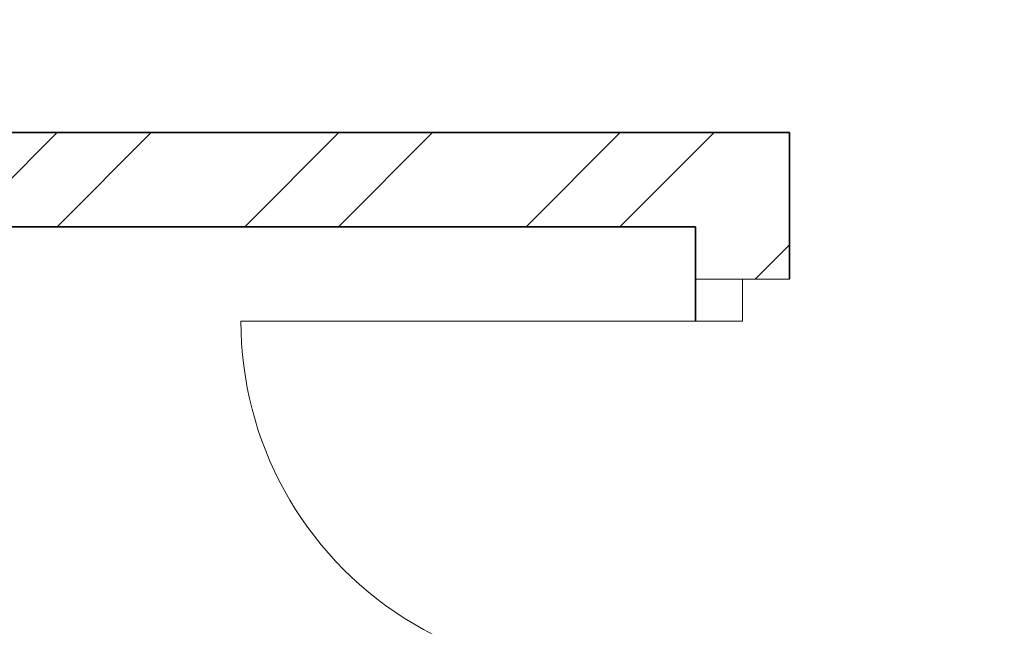
# Model space of a CAD drawing. Units: inches. Extents: x 1885 to 2748, y 783 to 2421.
# Tile 45 of 117: x 2192 to 2240, y 1591 to 1620. Entities that reach past the tile are written whole.
import ezdxf

# ---------------------------------------------------------------- set-up
doc = ezdxf.new("R2010")
doc.units = ezdxf.units.IN
doc.layers.add('A-DOOR', color=31, linetype='Continuous', lineweight=18)
doc.layers.add('A-WALL', color=7, linetype='Continuous', lineweight=35)
doc.layers.add('A-WALL-PATT', color=85, linetype='Continuous', lineweight=13, true_color=0x58ba48)

msp = doc.modelspace()

# ---------------------------------------------------------------- hatches: boundary and pattern name
at = {"layer": 'A-WALL-PATT'}
h = msp.add_hatch(dxfattribs=at)
h.set_pattern_fill('ANSI32', color=256)
h.paths.add_polyline_path([(2007.772, 2318.006), (1980.774, 2318.006), (1980.774, 2281.215), (1985.274, 2281.215), (1985.274, 2313.506), (2007.772, 2313.506), (2007.772, 2315.756)])
h.paths.add_polyline_path([(2094.324, 2318.006), (2067.772, 2318.006), (2067.772, 2313.506), (2094.324, 2313.506), (2094.324, 2315.756)])
h.paths.add_polyline_path([(2131.367, 2315.756), (2131.367, 2318.006), (2131.189, 2318.006), (2112.609, 2318.006), (2112.609, 2313.506), (2117.274, 2313.506), (2117.274, 2255.201), (2121.774, 2255.201), (2121.774, 2313.506), (2131.367, 2313.506)])
h.paths.add_polyline_path([(2190.512, 2318.006), (2155.367, 2318.006), (2155.367, 2313.506), (2169.774, 2313.506), (2169.774, 2229.506), (2121.774, 2229.506), (2121.774, 2233.451), (2119.524, 2233.451), (2117.274, 2233.451), (2117.274, 2201.101), (2121.774, 2201.101), (2121.774, 2225.006), (2169.774, 2225.006), (2169.774, 2165.006), (2306.274, 2165.006), (2306.274, 2066.006), (2310.774, 2066.006), (2344.274, 2066.006), (2486.274, 2066.006), (2486.274, 1886.006), (2483.02, 1886.006), (2483.02, 1881.506), (2486.274, 1881.506), (2486.274, 1880.678), (2490.774, 1880.678), (2490.774, 2070.506), (2344.274, 2070.506), (2310.774, 2070.506), (2310.774, 2165.006), (2310.774, 2173.636), (2308.524, 2173.636), (2306.274, 2173.636), (2306.274, 2169.506), (2174.274, 2169.506), (2174.274, 2313.506), (2190.512, 2313.506), (2190.512, 2315.756)])
h.paths.add_polyline_path([(1985.274, 2221.215), (1980.774, 2221.215), (1980.774, 2165.006), (1992.774, 2165.006), (1992.774, 2141.927), (1997.274, 2141.927), (1997.274, 2165.006), (2117.274, 2165.006), (2117.274, 2163.126), (2121.774, 2163.126), (2121.774, 2172.734), (2119.524, 2172.734), (2117.274, 2172.734), (2117.274, 2169.506), (1985.274, 2169.506)])
h.paths.add_polyline_path([(1997.274, 2105.927), (1992.774, 2105.927), (1992.774, 2070.506), (2016.774, 2070.506), (2016.774, 2059.123), (2019.024, 2059.123), (2021.274, 2059.123), (2021.274, 2070.506), (2117.274, 2070.506), (2117.274, 2022.506), (2114.423, 2022.506), (2114.423, 2018.006), (2123.627, 2018.006), (2123.627, 2020.256), (2123.627, 2022.506), (2121.774, 2022.506), (2121.774, 2142.587), (2119.524, 2142.587), (2117.274, 2142.587), (2117.274, 2075.006), (1997.274, 2075.006)])
h.paths.add_polyline_path([(2092.029, 2020.256), (2092.029, 2022.506), (2021.274, 2022.506), (2021.274, 2035.123), (2016.774, 2035.123), (2016.774, 2018.006), (2016.774, 1978.784), (2021.274, 1978.784), (2021.274, 2018.006), (2092.029, 2018.006)])
h.paths.add_polyline_path([(2260.938, 2022.506), (2153.105, 2022.506), (2153.105, 2020.256), (2153.105, 2018.006), (2155.274, 2018.006), (2155.274, 1886.006), (2107.629, 1886.006), (2107.629, 1881.506), (2182.911, 1881.506), (2182.911, 1883.756), (2182.911, 1886.006), (2159.774, 1886.006), (2159.774, 2018.006), (2260.938, 2018.006), (2260.938, 2020.256)])
h.paths.add_polyline_path([(2047.629, 1883.756), (2047.629, 1886.006), (2021.274, 1886.006), (2021.274, 1918.784), (2019.024, 1918.784), (2016.774, 1918.784), (2016.774, 1881.506), (2047.629, 1881.506)])
h.paths.add_polyline_path([(2306.361, 1883.756), (2306.361, 1886.006), (2296.274, 1886.006), (2296.274, 1982.006), (2316.535, 1982.006), (2316.535, 1984.256), (2316.535, 1986.506), (2296.274, 1986.506), (2296.274, 2022.506), (2289.276, 2022.506), (2289.276, 2018.006), (2291.774, 2018.006), (2291.774, 1886.006), (2242.911, 1886.006), (2242.911, 1881.506), (2306.361, 1881.506)], flags=17)
h.paths.add_polyline_path([(1985.274, 1843.006), (2021.6, 1843.006), (2021.534, 1845.441), (2021.477, 1847.506), (1980.774, 1847.506), (1980.774, 1809.446), (1985.274, 1809.446)])
h.paths.add_polyline_path([(2131.482, 1845.256), (2131.482, 1847.506), (2081.534, 1847.506), (2081.534, 1843.006), (2117.274, 1843.006), (2117.274, 1784.147), (2119.524, 1784.147), (2121.774, 1784.147), (2121.774, 1843.006), (2131.482, 1843.006)])
h.paths.add_polyline_path([(2203.886, 1847.506), (2155.482, 1847.506), (2155.482, 1843.006), (2169.774, 1843.006), (2169.774, 1759.006), (2121.774, 1759.006), (2121.774, 1761.457), (2117.274, 1761.457), (2117.274, 1730.429), (2121.774, 1730.429), (2121.774, 1754.506), (2177.421, 1754.506), (2177.421, 1756.756), (2177.421, 1759.006), (2174.274, 1759.006), (2174.274, 1843.006), (2203.886, 1843.006)])
h.paths.add_polyline_path([(2335.554, 1845.256), (2335.554, 1847.506), (2239.886, 1847.506), (2239.886, 1843.006), (2306.274, 1843.006), (2306.274, 1759.006), (2199.486, 1759.006), (2199.486, 1754.506), (2310.774, 1754.506), (2310.774, 1843.006), (2335.554, 1843.006)])
h.paths.add_polyline_path([(2348.774, 2022.506), (2344.274, 2022.506), (2344.274, 1986.506), (2341.681, 1986.506), (2341.681, 1982.006), (2344.274, 1982.006), (2344.274, 1886.006), (2330.361, 1886.006), (2330.361, 1881.506), (2361.627, 1881.506), (2361.627, 1883.756), (2361.627, 1886.006), (2348.774, 1886.006)], flags=17)
h.paths.add_polyline_path([(2283.251, 2315.756), (2283.251, 2318.006), (2238.512, 2318.006), (2238.512, 2313.506), (2283.251, 2313.506)], flags=17)
h.paths.add_polyline_path([(2363.274, 2348.006), (2388.677, 2348.006), (2388.677, 2350.256), (2388.677, 2352.506), (2358.774, 2352.506), (2358.774, 2348.006), (2358.774, 2318.006), (2344.481, 2318.006), (2344.481, 2313.506), (2358.774, 2313.506), (2358.774, 2229.506), (2310.774, 2229.506), (2310.774, 2231.952), (2306.274, 2231.952), (2306.274, 2205.611), (2310.774, 2205.611), (2310.774, 2225.006), (2358.774, 2225.006), (2358.774, 2211.506), (2452.329, 2211.506), (2452.329, 2213.756), (2452.329, 2216.006), (2363.274, 2216.006), (2363.274, 2318.006)])
h.paths.add_polyline_path([(2310.774, 2313.506), (2320.481, 2313.506), (2320.481, 2315.756), (2320.481, 2318.006), (2302.728, 2318.006), (2302.728, 2313.506), (2306.274, 2313.506), (2306.274, 2251.076), (2310.774, 2251.076)], flags=17)
h.paths.add_polyline_path([(2490.774, 2352.506), (2486.274, 2352.506), (2448.677, 2352.506), (2448.677, 2348.006), (2486.274, 2348.006), (2486.274, 2318.006), (2486.274, 2216.006), (2481.78, 2216.006), (2481.78, 2211.506), (2486.274, 2211.506), (2486.274, 2165.006), (2493.289, 2165.006), (2493.289, 2167.256), (2493.289, 2169.506), (2490.774, 2169.506), (2490.774, 2313.506), (2494.429, 2313.506), (2494.429, 2318.006), (2490.774, 2318.006)])
h.paths.add_polyline_path([(2534.653, 2318.006), (2515.691, 2318.006), (2515.691, 2313.506), (2534.653, 2313.506), (2534.653, 2315.756)])
h.paths.add_polyline_path([(2618.274, 2318.006), (2594.653, 2318.006), (2594.653, 2313.506), (2613.774, 2313.506), (2613.774, 2281.706), (2618.274, 2281.706)])
h.paths.add_polyline_path([(2618.274, 2221.706), (2613.774, 2221.706), (2613.774, 2169.506), (2554.019, 2169.506), (2554.019, 2165.006), (2613.774, 2165.006), (2613.774, 2152.878), (2618.274, 2152.878)])
h.paths.add_polyline_path([(2618.274, 2128.878), (2616.024, 2128.878), (2613.774, 2128.878), (2613.774, 2117.006), (2529.774, 2117.006), (2529.774, 2165.006), (2532.848, 2165.006), (2532.848, 2169.506), (2522.867, 2169.506), (2522.867, 2165.006), (2525.274, 2165.006), (2525.274, 2117.006), (2525.274, 2112.506), (2525.274, 2108.576), (2529.774, 2108.576), (2529.774, 2112.506), (2613.774, 2112.506), (2613.774, 2080.19), (2618.274, 2080.19)])
h.paths.add_polyline_path([(2618.274, 2044.19), (2616.024, 2044.19), (2613.774, 2044.19), (2613.774, 2015.506), (2529.774, 2015.506), (2529.774, 2088.582), (2527.524, 2088.582), (2525.274, 2088.582), (2525.274, 2011.006), (2613.774, 2011.006), (2613.774, 1956.755), (2618.274, 1956.755)])
h.paths.add_polyline_path([(2618.274, 1881.506), (2618.274, 1896.755), (2613.774, 1896.755), (2613.774, 1881.506), (2613.774, 1847.506), (2592.715, 1847.506), (2592.715, 1843.006), (2613.774, 1843.006), (2613.774, 1765.006), (2613.774, 1760.506), (2609.621, 1760.506), (2609.621, 1756.006), (2613.774, 1756.006), (2613.774, 1660.006), (2608.544, 1660.006), (2608.544, 1655.506), (2613.774, 1655.506), (2613.774, 1508.158), (2618.274, 1508.158)])
h.paths.add_polyline_path([(2565.774, 1843.006), (2568.997, 1843.006), (2568.997, 1847.506), (2490.774, 1847.506), (2490.774, 1849.7), (2488.524, 1849.7), (2486.274, 1849.7), (2486.274, 1847.506), (2477.274, 1847.506), (2477.274, 1838.506), (2477.274, 1821.493), (2486.274, 1821.493), (2486.274, 1838.506), (2561.274, 1838.506), (2561.274, 1765.006), (2486.274, 1765.006), (2486.274, 1786.157), (2477.274, 1786.157), (2477.274, 1765.006), (2477.274, 1756.006), (2486.274, 1756.006), (2565.774, 1756.006), (2585.621, 1756.006), (2585.621, 1758.256), (2585.621, 1760.506), (2565.774, 1760.506), (2565.774, 1765.006)])
h.paths.add_polyline_path([(2486.274, 1651.006), (2561.274, 1651.006), (2561.274, 1567.006), (2486.274, 1567.006), (2486.274, 1591.321), (2477.274, 1591.321), (2477.274, 1567.006), (2477.274, 1558.006), (2477.274, 1555.439), (2481.774, 1555.439), (2481.774, 1558.006), (2568.653, 1558.006), (2568.653, 1560.256), (2568.653, 1562.506), (2565.774, 1562.506), (2565.774, 1655.506), (2584.544, 1655.506), (2584.544, 1657.756), (2584.544, 1660.006), (2565.774, 1660.006), (2486.274, 1660.006), (2477.274, 1660.006), (2477.274, 1651.006), (2477.274, 1632.989), (2486.274, 1632.989)])
h.paths.add_polyline_path([(2449.967, 1883.756), (2449.967, 1886.006), (2421.627, 1886.006), (2421.627, 1881.506), (2449.967, 1881.506)], flags=17)
h.paths.add_polyline_path([(2447.274, 1847.506), (2395.554, 1847.506), (2395.554, 1843.006), (2442.774, 1843.006), (2442.774, 1809.27), (2447.274, 1809.27)])
h.paths.add_polyline_path([(1985.274, 1749.446), (1980.774, 1749.446), (1980.774, 1694.504), (1985.274, 1694.504), (1985.274, 1694.506), (1986.897, 1694.506), (1986.897, 1697.78), (1986.897, 1699.006), (1985.274, 1699.006)])
h.paths.add_polyline_path([(2152.774, 1699.006), (2121.774, 1699.006), (2121.774, 1703.668), (2119.524, 1703.668), (2117.274, 1703.668), (2117.274, 1699.006), (2009.219, 1699.006), (2009.219, 1694.506), (2148.274, 1694.506), (2148.274, 1692.631), (2152.774, 1692.631)])
h.paths.add_polyline_path([(2016.274, 1694.506), (2011.774, 1694.506), (2011.774, 1558.006), (2040.806, 1558.006), (2040.806, 1560.256), (2040.806, 1562.506), (2016.274, 1562.506)])
h.paths.add_polyline_path([(2152.774, 1663.017), (2150.524, 1663.017), (2148.274, 1663.017), (2148.274, 1562.506), (2100.806, 1562.506), (2100.806, 1558.006), (2165.119, 1558.006), (2165.119, 1560.256), (2165.119, 1562.506), (2152.774, 1562.506), (2152.774, 1610.506), (2224.774, 1610.506), (2224.774, 1607.99), (2229.274, 1607.99), (2229.274, 1615.006), (2152.774, 1615.006)])
h.paths.add_polyline_path([(2238.613, 1560.256), (2238.613, 1562.506), (2229.274, 1562.506), (2229.274, 1588.756), (2227.024, 1588.763), (2224.774, 1588.771), (2224.774, 1562.506), (2189.119, 1562.506), (2189.119, 1558.006), (2238.613, 1558.006)])
h.paths.add_polyline_path([(2336.024, 1560.256), (2336.024, 1562.506), (2310.774, 1562.506), (2310.774, 1656.347), (2308.524, 1656.347), (2306.274, 1656.347), (2306.274, 1562.506), (2286.613, 1562.506), (2286.613, 1558.006), (2336.024, 1558.006)])
h.paths.add_polyline_path([(2447.274, 1690.968), (2445.024, 1690.968), (2442.774, 1690.968), (2442.774, 1687.006), (2306.274, 1687.006), (2306.274, 1680.75), (2310.774, 1680.75), (2310.774, 1682.506), (2442.774, 1682.506), (2442.774, 1562.506), (2396.024, 1562.506), (2396.024, 1558.006), (2447.274, 1558.006)])
h.paths.add_polyline_path([(2447.274, 1749.27), (2445.024, 1749.27), (2442.774, 1749.27), (2442.774, 1717.232), (2447.274, 1717.232)])
h.paths.add_polyline_path([(2044.674, 1521.756), (2044.674, 1524.006), (2007.274, 1524.006), (2007.274, 1503.49), (2009.524, 1503.49), (2011.774, 1503.49), (2011.774, 1519.506), (2044.674, 1519.506)])
h.paths.add_polyline_path([(2177.969, 1521.756), (2177.969, 1524.006), (2104.674, 1524.006), (2104.674, 1519.506), (2145.774, 1519.506), (2145.774, 1387.506), (2143.37, 1387.506), (2143.37, 1383.006), (2251.585, 1383.006), (2251.585, 1385.256), (2251.585, 1387.506), (2150.274, 1387.506), (2150.274, 1519.506), (2177.969, 1519.506)])
h.paths.add_polyline_path([(2298.704, 1524.006), (2237.969, 1524.006), (2237.969, 1519.506), (2282.274, 1519.506), (2282.274, 1387.506), (2279.683, 1387.506), (2279.683, 1383.006), (2286.774, 1383.006), (2286.774, 1419.006), (2312.451, 1419.006), (2312.451, 1421.256), (2312.451, 1423.506), (2286.774, 1423.506), (2286.774, 1519.506), (2298.704, 1519.506), (2298.704, 1521.722)], flags=17)
h.paths.add_polyline_path([(2361.897, 1521.756), (2361.897, 1524.006), (2322.704, 1524.006), (2322.704, 1519.506), (2334.774, 1519.506), (2334.774, 1423.506), (2331.93, 1423.506), (2331.93, 1419.006), (2334.774, 1419.006), (2334.774, 1387.506), (2334.774, 1383.228), (2339.274, 1383.228), (2339.274, 1387.506), (2339.274, 1519.506), (2361.897, 1519.506)], flags=17)
h.paths.add_polyline_path([(2447.274, 1521.756), (2447.274, 1524.006), (2421.897, 1524.006), (2421.897, 1519.506), (2447.274, 1519.506)], flags=17)
h.paths.add_polyline_path([(2481.774, 1529.6), (2479.524, 1529.6), (2477.274, 1529.6), (2477.274, 1524.006), (2474.489, 1524.006), (2474.489, 1519.506), (2477.274, 1519.506), (2477.274, 1334.506), (2296.774, 1334.506), (2296.774, 1240.506), (2160.274, 1240.506), (2160.274, 1180.506), (2112.274, 1180.506), (2112.274, 1207.692), (2110.024, 1207.692), (2107.774, 1207.692), (2107.774, 1171.609), (2112.274, 1171.609), (2112.274, 1176.006), (2160.274, 1176.006), (2160.274, 1092.006), (2144.221, 1092.006), (2144.221, 1087.506), (2189.497, 1087.506), (2189.497, 1089.756), (2189.497, 1092.006), (2164.774, 1092.006), (2164.774, 1236.006), (2296.774, 1236.006), (2296.774, 1231.912), (2301.274, 1231.912), (2301.274, 1330.006), (2481.774, 1330.006), (2481.774, 1387.506)])
h.paths.add_polyline_path([(2618.274, 1448.158), (2613.774, 1448.158), (2613.774, 1382.506), (2529.774, 1382.506), (2525.274, 1382.506), (2525.274, 1307.062), (2529.774, 1307.062), (2529.774, 1378.006), (2613.774, 1378.006), (2613.774, 1354.988), (2618.274, 1354.988)])
h.paths.add_polyline_path([(2618.274, 1318.988), (2613.774, 1318.988), (2613.774, 1281.006), (2529.774, 1281.006), (2529.774, 1283.786), (2527.524, 1283.786), (2525.274, 1283.786), (2525.274, 1228.506), (2516.794, 1228.506), (2516.794, 1224.006), (2533.484, 1224.006), (2533.484, 1226.256), (2533.484, 1228.506), (2529.774, 1228.506), (2529.774, 1276.506), (2613.774, 1276.506), (2613.774, 1266.02), (2618.274, 1266.02)])
h.paths.add_polyline_path([(2618.274, 1134.964), (2613.774, 1134.964), (2613.774, 1092.006), (2594.545, 1092.006), (2594.545, 1087.506), (2618.274, 1087.506)])
h.paths.add_polyline_path([(2534.545, 1092.006), (2509.765, 1092.006), (2509.765, 1087.506), (2534.545, 1087.506), (2534.545, 1089.756)])
h.paths.add_polyline_path([(2481.274, 1224.006), (2484.117, 1224.006), (2484.117, 1226.256), (2484.117, 1228.506), (2476.774, 1228.506), (2476.774, 1198.506), (2471.61, 1198.506), (2471.61, 1194.006), (2476.774, 1194.006), (2476.774, 1062.006), (2436.894, 1062.006), (2436.894, 1057.506), (2476.774, 1057.506), (2481.274, 1057.506), (2481.274, 1062.006), (2481.274, 1087.506), (2485.354, 1087.506), (2485.354, 1089.756), (2485.354, 1092.006), (2481.274, 1092.006), (2481.274, 1117.506)])
h.paths.add_polyline_path([(2439.898, 1198.506), (2349.274, 1198.506), (2349.274, 1194.006), (2349.274, 1180.506), (2301.274, 1180.506), (2301.274, 1201.896), (2299.024, 1201.896), (2296.774, 1201.896), (2296.774, 1172.335), (2299.024, 1172.335), (2301.274, 1172.335), (2301.274, 1176.006), (2349.274, 1176.006), (2349.274, 1092.006), (2334.452, 1092.006), (2334.452, 1087.506), (2349.274, 1087.506), (2349.274, 1057.506), (2353.774, 1057.506), (2376.894, 1057.506), (2376.894, 1059.756), (2376.894, 1062.006), (2353.774, 1062.006), (2353.774, 1087.506), (2353.774, 1180.506), (2353.774, 1194.006), (2439.898, 1194.006), (2439.898, 1196.256)])
h.paths.add_polyline_path([(2270.596, 1089.756), (2270.596, 1092.006), (2249.497, 1092.006), (2249.497, 1087.506), (2270.596, 1087.506)], flags=17)
h.paths.add_polyline_path([(2310.452, 1092.006), (2301.274, 1092.006), (2301.274, 1153.292), (2296.774, 1153.292), (2296.774, 1092.006), (2293.786, 1092.006), (2293.786, 1087.506), (2310.452, 1087.506), (2310.452, 1089.756)], flags=17)
h.paths.add_polyline_path([(2112.274, 1150.328), (2110.024, 1150.328), (2107.774, 1150.328), (2107.774, 1092.006), (2104.465, 1092.006), (2104.465, 1087.506), (2120.221, 1087.506), (2120.221, 1089.756), (2120.221, 1092.006), (2112.274, 1092.006)])
h.paths.add_polyline_path([(2082.172, 1092.006), (2058.144, 1092.006), (2058.144, 1087.506), (2082.172, 1087.506), (2082.172, 1089.756)])
h.paths.add_polyline_path([(1975.774, 1145.638), (1971.274, 1145.638), (1971.274, 1087.506), (1980.774, 1087.506), (1998.144, 1087.506), (1998.144, 1089.756), (1998.144, 1092.006), (1985.274, 1092.006), (1975.774, 1092.006)])
h.paths.add_polyline_path([(2112.274, 1244.385), (2110.024, 1244.385), (2107.774, 1244.385), (2107.774, 1240.506), (1992.274, 1240.506), (1992.274, 1271.008), (1987.774, 1271.008), (1987.774, 1240.506), (1980.774, 1240.506), (1975.774, 1240.506), (1971.274, 1240.506), (1971.274, 1205.638), (1975.774, 1205.638), (1975.774, 1236.006), (2107.774, 1236.006), (2107.774, 1233.444), (2112.274, 1233.444), (2112.274, 1236.006)])
h.paths.add_polyline_path([(2112.274, 1383.006), (2114.783, 1383.006), (2114.783, 1385.256), (2114.783, 1387.506), (2102.476, 1387.506), (2102.476, 1383.006), (2107.774, 1383.006), (2107.774, 1335.006), (2011.774, 1335.006), (2011.774, 1349.939), (2007.274, 1349.939), (2007.274, 1335.006), (1987.774, 1335.006), (1987.774, 1330.506), (1987.774, 1307.008), (1992.274, 1307.008), (1992.274, 1330.506), (2007.274, 1330.506), (2107.774, 1330.506), (2107.774, 1264.711), (2112.274, 1264.711)])
h.paths.add_polyline_path([(2077.857, 1387.506), (2011.774, 1387.506), (2011.774, 1390.036), (2009.524, 1390.036), (2007.274, 1390.036), (2007.274, 1373.939), (2011.774, 1373.939), (2011.774, 1383.006), (2077.857, 1383.006)])
h.paths.add_polyline_path([(2011.774, 1443.49), (2007.274, 1443.49), (2007.274, 1410.248), (2011.774, 1410.248)])

# ---------------------------------------------------------------- linework, layer by layer
at = {"layer": 'A-DOOR'}
for p, q in [((2224.774, 1607.99), (2229.274, 1607.99)), ((2229.274, 1607.99), (2227.024, 1607.99)), ((2227.024, 1607.99), (2227.024, 1605.99)), ((2227.024, 1605.99), (2203.024, 1605.99))]:
    msp.add_line(p, q, dxfattribs=at)
msp.add_arc((2219.854, 1605.99), 16.83, 180, 295.2133, dxfattribs=at)
at = {"layer": 'A-WALL'}
for p, q in [((2152.774, 1615.006), (2229.274, 1615.006)), ((2229.274, 1615.006), (2229.274, 1607.99)), ((2152.774, 1610.506), (2224.774, 1610.506)), ((2224.774, 1610.506), (2224.774, 1605.99))]:
    msp.add_line(p, q, dxfattribs=at)

doc.saveas('drawing.dxf')
